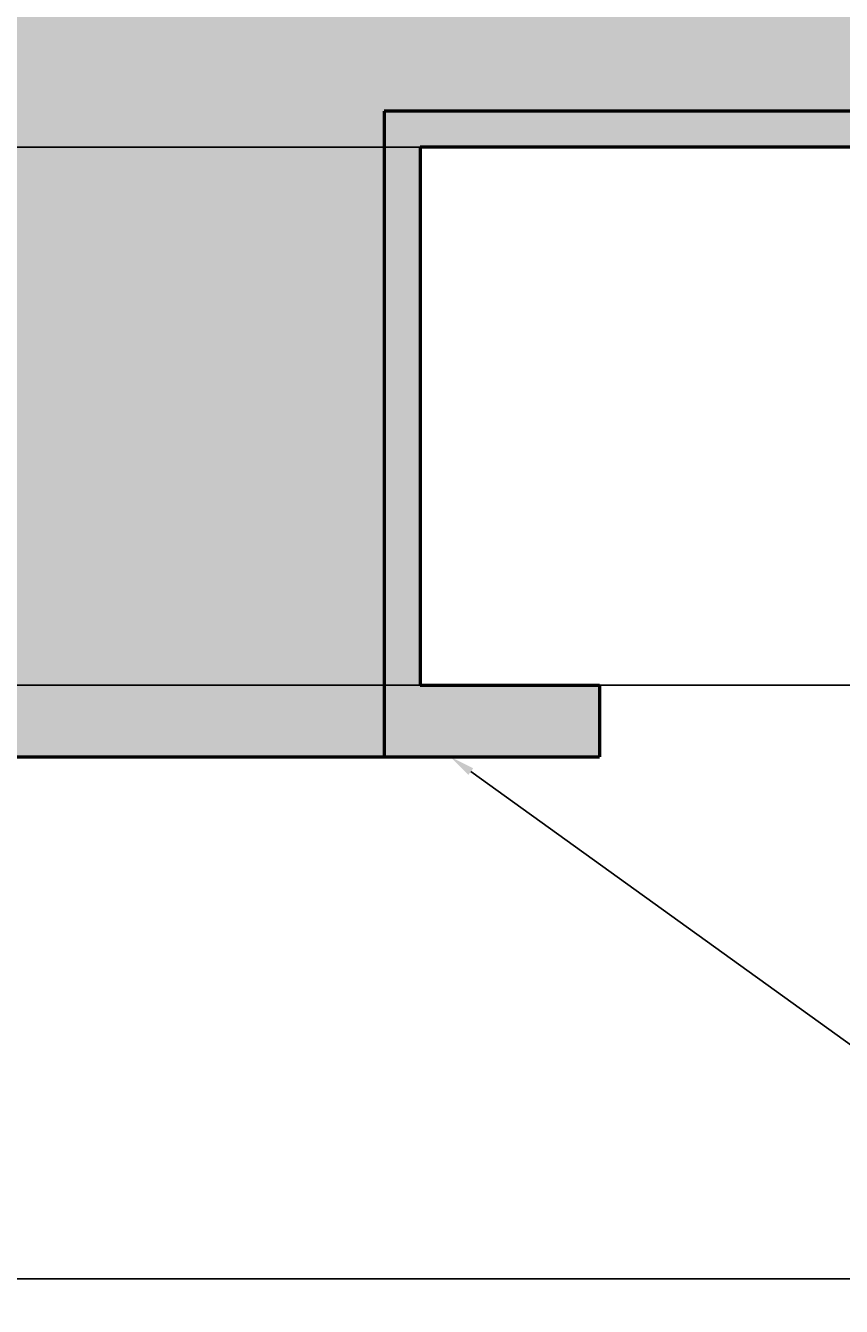
# Model space of a CAD drawing. Units: inches. Extents: x -12 to 334, y -10 to 186.
# Tile 30 of 77: x 106 to 129, y 14 to 49. Entities that reach past the tile are written whole.
import ezdxf
from ezdxf import colors
from ezdxf.entities.mleader import LeaderData, LeaderLine
from ezdxf.math import Vec2, Vec3

# ---------------------------------------------------------------- set-up
doc = ezdxf.new("R2010")
doc.units = ezdxf.units.IN
doc.header["$MEASUREMENT"] = 0
for name, color, linetype, lineweight in [('M-ANNO-TEXT', 3, 'Continuous', 25), ('M-DIMS', 2, 'Continuous', 18), ('M-EQPM', 7, 'Continuous', 50), ('M-EQPM-PATT', 8, 'Continuous', 18)]:
    doc.layers.add(name, color=color, linetype=linetype, lineweight=lineweight)
doc.styles.get("Standard").update_dxf_attribs({"font": 'arial.ttf'})
doc.dimstyles.get("Standard").update_dxf_attribs({"dimtxt": 0.18, "dimasz": 0.18, "dimexe": 0.18, "dimexo": 0.0625, "dimgap": 0.09, "dimtad": 0, "dimtih": 1, "dimtoh": 1, "dimdec": 4, "dimzin": 0, "dimdsep": 46, "dimtxsty": 'Standard', "dimcen": 0.09, "dimadec": 0, "dimazin": 0, "dimtfac": 1, "dimtdec": 4, "dimtofl": 0, "dimtmove": 0, "dimatfit": 3, "dimfxl": 1, "dimtolj": 1, "dimtzin": 0, "dimarcsym": 0})

# ---------------------------------------------------------------- blocks, each defined once
blk = doc.blocks.new('*D1')
at = {"layer": 'Defpoints', "color": 0, "transparency": 16777216}
for p in [(281.426, 91.899), (3.376, 80.692), (281.426, 14.304)]:
    blk.add_point(p, dxfattribs=at)
at = {"layer": 'M-DIMS', "color": 0, "lineweight": -2, "transparency": 16777216}
for p, q in [((281.426, 91.836), (281.426, 14.124)), ((3.376, 80.629), (3.376, 14.124)), ((3.556, 14.304), (141.935, 14.304)), ((281.246, 14.304), (142.867, 14.304))]:
    blk.add_line(p, q, dxfattribs=at)
at = {"layer": 'M-DIMS', "color": 0, "transparency": 16777216}
for points in [[(3.556, 14.334), (3.556, 14.274), (3.376, 14.304)], [(281.246, 14.334), (281.246, 14.274), (281.426, 14.304)]]:
    blk.add_solid(points, dxfattribs=at)
at = {"layer": 'M-DIMS', "color": 0, "transparency": 16777216, "insert": (142.401, 14.304), "char_height": 0.18, "attachment_point": 5}
blk.add_mtext('\\A1;278.05', dxfattribs=at)
blk = doc.blocks.new('*D29')
at = {"layer": 'Defpoints', "color": 0, "transparency": 16777216}
for p in [(-11.174, 45.854), (221.576, 45.854), (216.576, 30.854)]:
    blk.add_point(p, dxfattribs=at)
at = {"layer": 'M-DIMS', "color": 0, "lineweight": -2, "transparency": 16777216}
for p, q in [((221.514, 45.854), (-11.354, 45.854)), ((-11.174, 45.674), (-11.174, 38.536)), ((-11.174, 31.034), (-11.174, 38.172)), ((216.514, 30.854), (-11.354, 30.854))]:
    blk.add_line(p, q, dxfattribs=at)
at = {"layer": 'M-DIMS', "color": 0, "transparency": 16777216}
for points in [[(-11.204, 45.674), (-11.144, 45.674), (-11.174, 45.854)], [(-11.204, 31.034), (-11.144, 31.034), (-11.174, 30.854)]]:
    blk.add_solid(points, dxfattribs=at)
at = {"layer": 'M-DIMS', "color": 0, "transparency": 16777216, "insert": (-11.174, 38.354), "char_height": 0.18, "attachment_point": 5}
blk.add_mtext('\\A1;15', dxfattribs=at)
blk = doc.blocks.new('*D30')
at = {"layer": 'Defpoints', "color": 0, "transparency": 16777216}
for p in [(75.924, 63.612), (129.093, 61.105), (129.093, 14.304)]:
    blk.add_point(p, dxfattribs=at)
at = {"layer": 'M-DIMS', "color": 0, "lineweight": -2, "transparency": 16777216}
for p, q in [((75.924, 63.549), (75.924, 14.124)), ((129.093, 61.042), (129.093, 14.124)), ((76.104, 14.304), (102.115, 14.304)), ((128.913, 14.304), (102.902, 14.304))]:
    blk.add_line(p, q, dxfattribs=at)
at = {"layer": 'M-DIMS', "color": 0, "transparency": 16777216}
for points in [[(76.104, 14.334), (76.104, 14.274), (75.924, 14.304)], [(128.913, 14.334), (128.913, 14.274), (129.093, 14.304)]]:
    blk.add_solid(points, dxfattribs=at)
at = {"layer": 'M-DIMS', "color": 0, "transparency": 16777216, "insert": (102.509, 14.304), "char_height": 0.18, "attachment_point": 5}
blk.add_mtext('\\A1;53.17', dxfattribs=at)
blk = doc.blocks.new('*D39')
at = {"layer": 'Defpoints', "color": 0, "transparency": 16777216}
for p in [(279.726, 80.692), (-11.174, 45.854), (269.381, 45.854)]:
    blk.add_point(p, dxfattribs=at)
at = {"layer": 'M-DIMS', "color": 0, "lineweight": -2, "transparency": 16777216}
for p, q in [((279.664, 80.692), (-11.354, 80.692)), ((-11.174, 80.512), (-11.174, 63.455)), ((-11.174, 46.034), (-11.174, 63.091)), ((269.318, 45.854), (-11.354, 45.854))]:
    blk.add_line(p, q, dxfattribs=at)
at = {"layer": 'M-DIMS', "color": 0, "transparency": 16777216}
for points in [[(-11.204, 80.512), (-11.144, 80.512), (-11.174, 80.692)], [(-11.204, 46.034), (-11.144, 46.034), (-11.174, 45.854)]]:
    blk.add_solid(points, dxfattribs=at)
at = {"layer": 'M-DIMS', "color": 0, "transparency": 16777216, "insert": (-11.174, 63.273), "char_height": 0.18, "attachment_point": 5}
blk.add_mtext('\\A1;34.84', dxfattribs=at)

msp = doc.modelspace()

# ---------------------------------------------------------------- hatches: boundary and pattern name
at = {"layer": 'M-EQPM-PATT'}
h = msp.add_hatch(color=256, dxfattribs=at)
h.set_gradient(color1=(99, 100, 102), color2=(99, 100, 102), tint=1)
h.paths.add_polyline_path([(4.3766, 80.754, -0.4132606), (23.5807, 99.8958), (37.1002, 99.8958), (37.1002, 127.7078), (32.1002, 127.7078), (32.1002, 125.2078), (36.1002, 125.2078), (36.1002, 100.8958), (23.5807, 100.8958, 1), (23.5807, 60.4872), (36.1002, 60.4872), (36.1002, 36.1752), (32.1002, 36.1752), (32.1002, 33.6752), (37.1002, 33.6752), (37.1002, 61.4872), (23.5807, 61.4872, -0.384914), (4.4744, 78.754), (72.9244, 78.754), (72.9244, 69.6117), (75.9244, 69.6117), (75.9244, 89.8963), (72.9244, 89.8963), (72.9244, 80.754)])
h.paths.add_polyline_path([(54.1002, 125.2078), (58.1002, 125.2078), (58.1002, 127.7078), (53.1002, 127.7078), (53.1002, 99.8958), (64.5, 99.8958), (64.5, 109.0583), (63.5, 109.0583), (63.5, 100.8958), (54.1002, 100.8958)], flags=17)
h.paths.add_polyline_path([(53.1002, 33.6752), (58.1002, 33.6752), (58.1002, 36.1752), (54.1002, 36.1752), (54.1002, 60.4872), (64.2068, 60.4872), (64.2068, 49.4497), (87.8879, 49.4497), (87.8879, 55.3205), (104.8919, 55.3205), (104.8919, 30.8541), (99.8919, 30.8541), (99.8919, 28.8541), (105.8919, 28.8541), (105.8919, 56.3205), (87.8879, 56.3205), (87.8879, 63.6117), (86.8879, 63.6117), (86.8879, 50.4497), (65.0061, 50.4497), (65.0061, 63.6117), (64.5, 63.6117), (64.5, 61.4872), (53.1002, 61.4872)])
h.paths.add_polyline_path([(121.8919, 28.8541), (121.8919, 30.8541), (116.8919, 30.8541), (116.8919, 45.8541), (209.6965, 45.8541), (209.9204, 46.8541), (115.8919, 46.8541), (115.8919, 28.8541)])
h.paths.add_polyline_path([(221.5761, 32.8541), (216.5761, 32.8541), (216.5761, 30.8541), (222.5761, 30.8541), (222.5761, 46.8541), (209.9204, 46.8541), (209.6965, 45.8541), (221.5761, 45.8541)])
h.paths.add_polyline_path([(233.5761, 45.8541), (249.8485, 45.8541), (249.3759, 46.8541), (232.5761, 46.8541), (232.5761, 30.8541), (238.5761, 30.8541), (238.5761, 32.8541), (233.5761, 32.8541)])
h = msp.add_hatch(color=256, dxfattribs=at)
h.set_gradient(color1=(94, 103, 175), color2=(94, 103, 175), tint=1)
h.paths.add_polyline_path([(129.093, 89.8963), (86.8879, 89.8963), (86.8879, 69.6117), (129.093, 69.6117)], flags=17)
h.paths.add_polyline_path([(170.9079, 89.8963), (130.8573, 89.8963), (130.8573, 69.6117), (170.9079, 69.6117)], flags=17)
h.paths.add_polyline_path([(216.4278, 89.8963), (172.6722, 89.8963), (172.6722, 69.6117), (216.4278, 69.6117)], flags=17)
h.paths.add_polyline_path([(245.9354, 82.6969), (247.9354, 82.6969), (247.9354, 46.8541), (268.3808, 46.8541, 0.0998398), (279.7263, 80.6915), (251.9801, 80.6915, 0.4142136), (231.7758, 100.8958), (84.7229, 100.8958), (84.7229, 109.0583), (83.7229, 109.0583), (83.7229, 95.8963), (129.093, 95.8963), (129.093, 98.1081), (130.8573, 98.1081), (130.8573, 95.8963), (170.9079, 95.8963), (170.9079, 98.1081), (172.6722, 98.1081), (172.6722, 95.8963), (216.4278, 95.8963), (216.4278, 98.1081), (218.1922, 98.1081), (218.1922, 95.8963), (226.6083, 95.8963, -1), (226.6083, 63.6117), (218.1922, 63.6117), (218.1922, 61.1045), (216.4278, 61.1045), (216.4278, 63.6117), (172.6722, 63.6117), (172.6722, 61.1045), (170.9079, 61.1045), (170.9079, 63.6117), (130.8573, 63.6117), (130.8573, 61.1045), (129.093, 61.1045), (129.093, 63.6117), (87.8879, 63.6117), (87.8879, 56.3205), (105.8919, 56.3205), (105.8919, 28.8541), (115.8919, 28.8541), (115.8919, 46.8541), (222.5761, 46.8541), (222.5761, 30.8541), (232.5761, 30.8541), (232.5761, 46.8541), (245.9354, 46.8541)])
h.paths.add_polyline_path([(86.8879, 89.8963), (75.9244, 89.8963), (75.9244, 69.6117), (86.8879, 69.6117)])
h.paths.add_polyline_path([(83.7229, 109.0583), (75.9244, 109.0583), (75.9244, 95.8963), (83.7229, 95.8963)])
h.paths.add_polyline_path([(226.6083, 89.8963), (218.1922, 89.8963), (218.1922, 69.6117), (226.6083, 69.6117, 1)], flags=17)
h = msp.add_hatch(color=256, dxfattribs=at)
h.set_gradient(color1=(0, 0, 255), color2=(0, 0, 255), tint=1)
h.paths.add_polyline_path([(84.7229, 100.8958), (84.7229, 109.0583), (83.7229, 109.0583), (83.7229, 95.8963), (129.093, 95.8963), (129.093, 98.1081), (130.8573, 98.1081), (130.8573, 95.8963), (170.9079, 95.8963), (170.9079, 98.1081), (172.6722, 98.1081), (172.6722, 95.8963), (216.4278, 95.8963), (216.4278, 98.1081), (218.1922, 98.1081), (218.1922, 95.8963), (226.6083, 95.8963, -1), (226.6083, 63.6117), (218.1922, 63.6117), (218.1922, 61.1045), (216.4278, 61.1045), (216.4278, 63.6117), (172.6722, 63.6117), (172.6722, 61.1045), (170.9079, 61.1045), (170.9079, 63.6117), (130.8573, 63.6117), (130.8573, 61.1045), (129.093, 61.1045), (129.093, 63.6117), (87.8879, 63.6117), (87.8879, 56.3205), (105.8919, 56.3205), (105.8919, 28.8541), (115.8919, 28.8541), (115.8919, 46.8541), (222.5761, 46.8541), (222.5761, 30.8541), (232.5761, 30.8541), (232.5761, 46.8541), (245.9354, 46.8541), (245.9354, 82.6969), (247.9354, 82.6969), (247.9354, 46.8541), (268.3808, 46.8541, 0.0998398), (279.7263, 80.6915), (251.9801, 80.6915, 0.4142136), (231.7758, 100.8958)])

# ---------------------------------------------------------------- linework, layer by layer
at = {"layer": 'M-EQPM'}
for p, q in [((222.5761, 46.8541), (115.8919, 46.8541)), ((115.8919, 46.8541), (115.8919, 28.8541)), ((221.5761, 45.8541), (116.8919, 45.8541)), ((116.8919, 45.8541), (116.8919, 30.8541)), ((116.8919, 30.8541), (121.8919, 30.8541)), ((121.8919, 30.8541), (121.8919, 28.8541)), ((99.8919, 28.8541), (121.8919, 28.8541))]:
    msp.add_line(p, q, dxfattribs=at)

# ---------------------------------------------------------------- dimensions: what is measured, and where the dimension line sits
at = {"layer": 'M-DIMS'}
for base, p1, p2, picture, middle in [((281.4256, 14.3041), (3.3765, 80.6915), (281.4256, 91.8988), '*D1', (142.401, 14.3041)), ((129.093, 14.3041), (75.9244, 63.6117), (129.093, 61.1045), '*D30', (102.5087, 14.3041))]:
    dim = msp.add_linear_dim(base=base, p1=p1, p2=p2, dimstyle='Standard', override={"dimdec": 2, "dimlfac": 1, "dimrnd": 0, "dimzin": 0, "dimdsep": 46, "dimlunit": 2}, dxfattribs=at)
    dim.commit()
    dim.dimension.update_dxf_attribs({"geometry": picture, "text_midpoint": middle})
for p1, p2, override, picture, middle in [((279.7263, 80.6915), (269.3808, 45.8541), {"dimdec": 2, "dimlfac": 1, "dimrnd": 0, "dimzin": 0, "dimdsep": 46, "dimlunit": 2}, '*D39', (-11.1735, 63.2728)), ((216.5761, 30.8541), (221.5761, 45.8541), {"dimdec": 0, "dimlfac": 1, "dimrnd": 0, "dimzin": 0, "dimdsep": 46, "dimlunit": 2}, '*D29', (-11.1735, 38.3541))]:
    dim = msp.add_linear_dim(base=(-11.1736, 45.8541), p1=p1, p2=p2, angle=90, dimstyle='Standard', override=override, dxfattribs=at)
    dim.commit()
    dim.dimension.update_dxf_attribs({"geometry": picture, "text_midpoint": middle})

# ---------------------------------------------------------------- leaders
at = {"layer": 'M-ANNO-TEXT'}
ml = msp.add_multileader_mtext('Standard', dxfattribs=at)
ml.set_content('^ICondensate outlet', color=256)
ml.set_leader_properties()
ml.build(insert=Vec2(0, 0))
ml.multileader.update_dxf_attribs({"dogleg_length": 0.36, "arrow_head_size": 0.7})
ctx = ml.context
ctx.base_point, ctx.arrow_head_size, ctx.landing_gap_size, ctx.plane_origin = Vec3(83.8784, 10.3512), 0.7, 0.09, Vec3(49.4251, 25.7584)
notes = []
notes.append((ctx, [(0, (1, 1, 0), (70.8242, 10.3512), (1, 0), 13.0542, [(0, [(42.9275, 33.6752)], 0, [])])]))
ctx.mtext.insert, ctx.mtext.flow_direction = Vec3(83.9684, 12.3853), 5
ml = msp.add_multileader_mtext('Standard', dxfattribs=at)
ml.set_content('liquid feed from\\Pcolumn', color=256)
ml.set_leader_properties()
ml.build(insert=Vec2(0, 0))
ml.multileader.update_dxf_attribs({"dogleg_length": 0.36, "arrow_head_size": 0.7})
ctx = ml.context
ctx.base_point, ctx.arrow_head_size, ctx.landing_gap_size, ctx.plane_origin = Vec3(152.1867, 13.4469), 0.7, 0.09, Vec3(117.7335, 28.8541)
notes.append((ctx, [(0, (1, 1, 0), (139.1325, 13.4469), (1, 0), 13.0542, [(0, [(117.7335, 28.8541)], 0, [])])]))
ctx.mtext.insert, ctx.mtext.flow_direction = Vec3(152.2767, 15.4796), 5
for ctx, leaders in notes:
    for number, flags, end, landing, length, lines in leaders:
        leader = LeaderData()
        leader.index, (leader.has_last_leader_line, leader.has_dogleg_vector, leader.attachment_direction) = number, flags
        leader.last_leader_point, leader.dogleg_vector, leader.dogleg_length = Vec3(end), Vec3(landing), length
        for number, points, colour, breaks in lines:
            line = LeaderLine()
            line.index, line.vertices, line.color, line.breaks = number, Vec3.list(points), colors.encode_raw_color(colour), breaks
            leader.lines.append(line)
        ctx.leaders.append(leader)

doc.saveas('drawing.dxf')
